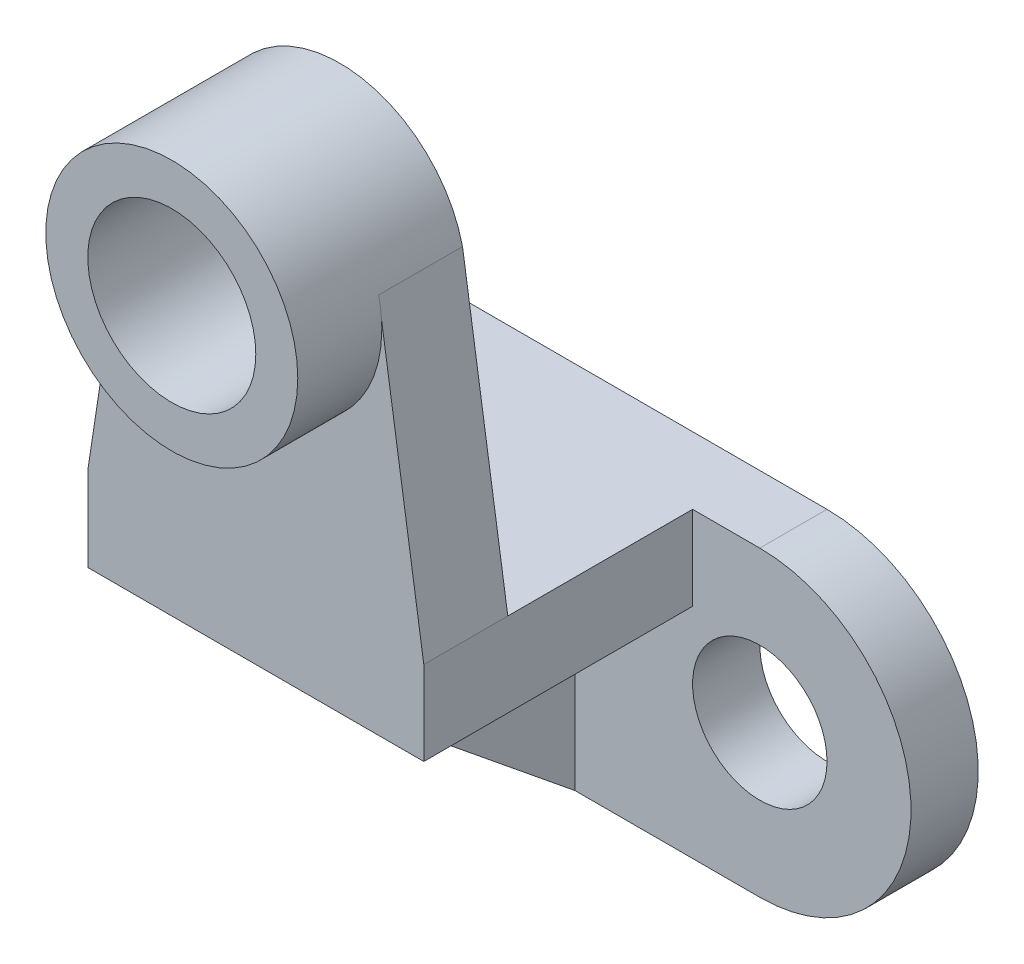
ISO-10303-21;
HEADER;
FILE_DESCRIPTION(('STEP AP214'),'2;1');
FILE_NAME('part.step','',(''),(''),'','','');
FILE_SCHEMA(('AUTOMOTIVE_DESIGN { 1 0 10303 214 1 1 1 1 }'));
ENDSEC;
DATA;
#1=APPLICATION_CONTEXT('core data for automotive mechanical design processes');
#2=APPLICATION_PROTOCOL_DEFINITION('international standard','automotive_design',2000,#1);
#3=PRODUCT_CONTEXT('',#1,'mechanical');
#4=PRODUCT('Part','Part','',(#3));
#5=PRODUCT_RELATED_PRODUCT_CATEGORY('part','',(#4));
#6=PRODUCT_DEFINITION_FORMATION('','',#4);
#7=PRODUCT_DEFINITION_CONTEXT('part definition',#1,'design');
#8=PRODUCT_DEFINITION('design','',#6,#7);
#9=PRODUCT_DEFINITION_SHAPE('','',#8);
#10=(LENGTH_UNIT() NAMED_UNIT(*) SI_UNIT(.MILLI.,.METRE.));
#11=(NAMED_UNIT(*) PLANE_ANGLE_UNIT() SI_UNIT($,.RADIAN.));
#12=(NAMED_UNIT(*) SI_UNIT($,.STERADIAN.) SOLID_ANGLE_UNIT());
#13=UNCERTAINTY_MEASURE_WITH_UNIT(LENGTH_MEASURE(1.E-05),#10,'distance_accuracy_value','');
#14=(GEOMETRIC_REPRESENTATION_CONTEXT(3) GLOBAL_UNCERTAINTY_ASSIGNED_CONTEXT((#13)) GLOBAL_UNIT_ASSIGNED_CONTEXT((#10,
#11,#12)) REPRESENTATION_CONTEXT('',''));
#15=CARTESIAN_POINT('',(0.,0.,0.));
#16=DIRECTION('',(0.,0.,1.));
#17=DIRECTION('',(1.,0.,0.));
#18=AXIS2_PLACEMENT_3D('',#15,#16,#17);
#19=CARTESIAN_POINT('',(8.,8.,40.));
#20=DIRECTION('',(0.,-0.776114000116266,0.630592625094466));
#21=DIRECTION('',(0.,-0.630592625094466,-0.776114000116266));
#22=AXIS2_PLACEMENT_3D('',#19,#20,#21);
#23=PLANE('',#22);
#24=DIRECTION('',(0.,0.630592625094466,0.776114000116266));
#25=VECTOR('',#24,1.);
#26=CARTESIAN_POINT('',(22.,-18.,8.));
#27=LINE('',#26,#25);
#28=CARTESIAN_POINT('',(22.,-18.,8.));
#29=VERTEX_POINT('',#28);
#30=CARTESIAN_POINT('',(22.,8.,40.));
#31=VERTEX_POINT('',#30);
#32=EDGE_CURVE('E63',#29,#31,#27,.T.);
#33=ORIENTED_EDGE('',*,*,#32,.F.);
#34=DIRECTION('',(1.,0.,0.));
#35=VECTOR('',#34,1.);
#36=CARTESIAN_POINT('',(8.,-18.,8.));
#37=LINE('',#36,#35);
#38=CARTESIAN_POINT('',(34.,-18.,8.));
#39=VERTEX_POINT('',#38);
#40=EDGE_CURVE('E194',#29,#39,#37,.T.);
#41=ORIENTED_EDGE('',*,*,#40,.T.);
#42=DIRECTION('',(0.,-0.630592625094466,-0.776114000116266));
#43=VECTOR('',#42,1.);
#44=CARTESIAN_POINT('',(34.,-18.,8.));
#45=LINE('',#44,#43);
#46=CARTESIAN_POINT('',(34.,8.,40.));
#47=VERTEX_POINT('',#46);
#48=EDGE_CURVE('E181',#47,#39,#45,.T.);
#49=ORIENTED_EDGE('',*,*,#48,.F.);
#50=DIRECTION('',(1.,0.,0.));
#51=VECTOR('',#50,1.);
#52=CARTESIAN_POINT('',(8.,8.,40.));
#53=LINE('',#52,#51);
#54=EDGE_CURVE('E75',#31,#47,#53,.T.);
#55=ORIENTED_EDGE('',*,*,#54,.F.);
#56=EDGE_LOOP('',(#33,#41,#49,#55));
#57=FACE_BOUND('',#56,.T.);
#58=ADVANCED_FACE('F50',(#57),#23,.T.);
#59=CARTESIAN_POINT('',(0.,0.,8.));
#60=DIRECTION('',(0.,0.,1.));
#61=DIRECTION('',(1.,0.,0.));
#62=AXIS2_PLACEMENT_3D('',#59,#60,#61);
#63=PLANE('',#62);
#64=DIRECTION('',(0.,1.,0.));
#65=VECTOR('',#64,1.);
#66=CARTESIAN_POINT('',(48.,8.,8.));
#67=LINE('',#66,#65);
#68=CARTESIAN_POINT('',(48.,8.00000000000001,8.));
#69=VERTEX_POINT('',#68);
#70=CARTESIAN_POINT('',(48.,18.,8.));
#71=VERTEX_POINT('',#70);
#72=EDGE_CURVE('E235',#69,#71,#67,.T.);
#73=ORIENTED_EDGE('',*,*,#72,.F.);
#74=DIRECTION('',(1.,0.,0.));
#75=VECTOR('',#74,1.);
#76=CARTESIAN_POINT('',(34.,8.00000000000001,8.));
#77=LINE('',#76,#75);
#78=CARTESIAN_POINT('',(34.,8.00000000000001,8.));
#79=VERTEX_POINT('',#78);
#80=EDGE_CURVE('E186',#79,#69,#77,.T.);
#81=ORIENTED_EDGE('',*,*,#80,.F.);
#82=DIRECTION('',(0.,1.,0.));
#83=VECTOR('',#82,1.);
#84=CARTESIAN_POINT('',(34.,8.00000000000001,8.));
#85=LINE('',#84,#83);
#86=EDGE_CURVE('E183',#39,#79,#85,.T.);
#87=ORIENTED_EDGE('',*,*,#86,.F.);
#88=DIRECTION('',(1.,0.,0.));
#89=VECTOR('',#88,1.);
#90=CARTESIAN_POINT('',(56.,-18.,8.));
#91=LINE('',#90,#89);
#92=CARTESIAN_POINT('',(56.,-18.,8.));
#93=VERTEX_POINT('',#92);
#94=EDGE_CURVE('E264',#39,#93,#91,.T.);
#95=ORIENTED_EDGE('',*,*,#94,.T.);
#96=CARTESIAN_POINT('',(56.,0.,8.));
#97=DIRECTION('',(0.,0.,1.));
#98=DIRECTION('',(1.,0.,0.));
#99=AXIS2_PLACEMENT_3D('',#96,#97,#98);
#100=CIRCLE('',#99,18.);
#101=CARTESIAN_POINT('',(56.,18.,8.));
#102=VERTEX_POINT('',#101);
#103=EDGE_CURVE('E263',#93,#102,#100,.T.);
#104=ORIENTED_EDGE('',*,*,#103,.T.);
#105=DIRECTION('',(-1.,0.,0.));
#106=VECTOR('',#105,1.);
#107=CARTESIAN_POINT('',(0.,18.,8.));
#108=LINE('',#107,#106);
#109=EDGE_CURVE('E270',#102,#71,#108,.T.);
#110=ORIENTED_EDGE('',*,*,#109,.T.);
#111=EDGE_LOOP('',(#73,#81,#87,#95,#104,#110));
#112=FACE_BOUND('',#111,.T.);
#113=CARTESIAN_POINT('',(56.,0.,8.));
#114=DIRECTION('',(0.,0.,1.));
#115=DIRECTION('',(1.,0.,0.));
#116=AXIS2_PLACEMENT_3D('',#113,#114,#115);
#117=CIRCLE('',#116,8.00000000000001);
#118=CARTESIAN_POINT('',(64.,0.,8.));
#119=VERTEX_POINT('',#118);
#120=EDGE_CURVE('E250',#119,#119,#117,.T.);
#121=ORIENTED_EDGE('',*,*,#120,.F.);
#122=EDGE_LOOP('',(#121));
#123=FACE_BOUND('',#122,.T.);
#124=ADVANCED_FACE('F311',(#112,#123),#63,.T.);
#125=CARTESIAN_POINT('',(0.,18.,8.));
#126=DIRECTION('',(0.,-1.,0.));
#127=DIRECTION('',(1.,0.,0.));
#128=AXIS2_PLACEMENT_3D('',#125,#126,#127);
#129=PLANE('',#128);
#130=DIRECTION('',(-1.,0.,0.));
#131=VECTOR('',#130,1.);
#132=CARTESIAN_POINT('',(0.,18.,30.));
#133=LINE('',#132,#131);
#134=CARTESIAN_POINT('',(48.,18.,30.));
#135=VERTEX_POINT('',#134);
#136=CARTESIAN_POINT('',(8.,18.,30.));
#137=VERTEX_POINT('',#136);
#138=EDGE_CURVE('E217',#135,#137,#133,.T.);
#139=ORIENTED_EDGE('',*,*,#138,.F.);
#140=DIRECTION('',(0.,0.,-1.));
#141=VECTOR('',#140,1.);
#142=CARTESIAN_POINT('',(48.,18.,40.));
#143=LINE('',#142,#141);
#144=EDGE_CURVE('E238',#135,#71,#143,.T.);
#145=ORIENTED_EDGE('',*,*,#144,.T.);
#146=ORIENTED_EDGE('',*,*,#109,.F.);
#147=DIRECTION('',(0.,0.,-1.));
#148=VECTOR('',#147,1.);
#149=CARTESIAN_POINT('',(56.,18.,8.));
#150=LINE('',#149,#148);
#151=CARTESIAN_POINT('',(56.,18.,0.));
#152=VERTEX_POINT('',#151);
#153=EDGE_CURVE('E282',#102,#152,#150,.T.);
#154=ORIENTED_EDGE('',*,*,#153,.T.);
#155=DIRECTION('',(-1.,0.,0.));
#156=VECTOR('',#155,1.);
#157=CARTESIAN_POINT('',(0.,18.,0.));
#158=LINE('',#157,#156);
#159=CARTESIAN_POINT('',(0.,18.,0.));
#160=VERTEX_POINT('',#159);
#161=EDGE_CURVE('E265',#152,#160,#158,.T.);
#162=ORIENTED_EDGE('',*,*,#161,.T.);
#163=DIRECTION('',(0.,0.,-1.));
#164=VECTOR('',#163,1.);
#165=CARTESIAN_POINT('',(0.,18.,8.));
#166=LINE('',#165,#164);
#167=CARTESIAN_POINT('',(0.,18.,8.));
#168=VERTEX_POINT('',#167);
#169=EDGE_CURVE('E272',#168,#160,#166,.T.);
#170=ORIENTED_EDGE('',*,*,#169,.F.);
#171=CARTESIAN_POINT('',(8.,18.,8.));
#172=VERTEX_POINT('',#171);
#173=EDGE_CURVE('E266',#172,#168,#108,.T.);
#174=ORIENTED_EDGE('',*,*,#173,.F.);
#175=DIRECTION('',(0.,0.,-1.));
#176=VECTOR('',#175,1.);
#177=CARTESIAN_POINT('',(8.,18.,40.));
#178=LINE('',#177,#176);
#179=EDGE_CURVE('E243',#137,#172,#178,.T.);
#180=ORIENTED_EDGE('',*,*,#179,.F.);
#181=EDGE_LOOP('',(#139,#145,#146,#154,#162,#170,#174,#180));
#182=FACE_BOUND('',#181,.T.);
#183=ADVANCED_FACE('F306',(#182),#129,.F.);
#184=CARTESIAN_POINT('',(0.,0.,8.));
#185=DIRECTION('',(0.,0.,-1.));
#186=DIRECTION('',(-1.,0.,0.));
#187=AXIS2_PLACEMENT_3D('',#184,#185,#186);
#188=CYLINDRICAL_SURFACE('',#187,18.);
#189=CARTESIAN_POINT('',(0.,0.,0.));
#190=DIRECTION('',(0.,0.,1.));
#191=DIRECTION('',(1.,0.,0.));
#192=AXIS2_PLACEMENT_3D('',#189,#190,#191);
#193=CIRCLE('',#192,18.);
#194=CARTESIAN_POINT('',(0.,-18.,0.));
#195=VERTEX_POINT('',#194);
#196=EDGE_CURVE('E252',#160,#195,#193,.T.);
#197=ORIENTED_EDGE('',*,*,#196,.T.);
#198=DIRECTION('',(0.,0.,-1.));
#199=VECTOR('',#198,1.);
#200=CARTESIAN_POINT('',(0.,-18.,8.));
#201=LINE('',#200,#199);
#202=CARTESIAN_POINT('',(0.,-18.,8.));
#203=VERTEX_POINT('',#202);
#204=EDGE_CURVE('E51',#203,#195,#201,.T.);
#205=ORIENTED_EDGE('',*,*,#204,.F.);
#206=CARTESIAN_POINT('',(0.,0.,8.));
#207=DIRECTION('',(0.,0.,1.));
#208=DIRECTION('',(1.,0.,0.));
#209=AXIS2_PLACEMENT_3D('',#206,#207,#208);
#210=CIRCLE('',#209,18.);
#211=EDGE_CURVE('E258',#168,#203,#210,.T.);
#212=ORIENTED_EDGE('',*,*,#211,.F.);
#213=ORIENTED_EDGE('',*,*,#169,.T.);
#214=EDGE_LOOP('',(#197,#205,#212,#213));
#215=FACE_BOUND('',#214,.T.);
#216=ADVANCED_FACE('F47',(#215),#188,.T.);
#217=CARTESIAN_POINT('',(56.,-18.,8.));
#218=DIRECTION('',(0.,1.,0.));
#219=DIRECTION('',(-1.,0.,0.));
#220=AXIS2_PLACEMENT_3D('',#217,#218,#219);
#221=PLANE('',#220);
#222=DIRECTION('',(1.,0.,0.));
#223=VECTOR('',#222,1.);
#224=CARTESIAN_POINT('',(56.,-18.,0.));
#225=LINE('',#224,#223);
#226=CARTESIAN_POINT('',(56.,-18.,0.));
#227=VERTEX_POINT('',#226);
#228=EDGE_CURVE('E274',#195,#227,#225,.T.);
#229=ORIENTED_EDGE('',*,*,#228,.T.);
#230=DIRECTION('',(0.,0.,-1.));
#231=VECTOR('',#230,1.);
#232=CARTESIAN_POINT('',(56.,-18.,8.));
#233=LINE('',#232,#231);
#234=EDGE_CURVE('E285',#93,#227,#233,.T.);
#235=ORIENTED_EDGE('',*,*,#234,.F.);
#236=ORIENTED_EDGE('',*,*,#94,.F.);
#237=ORIENTED_EDGE('',*,*,#40,.F.);
#238=EDGE_CURVE('E176',#203,#29,#91,.T.);
#239=ORIENTED_EDGE('',*,*,#238,.F.);
#240=ORIENTED_EDGE('',*,*,#204,.T.);
#241=EDGE_LOOP('',(#229,#235,#236,#237,#239,#240));
#242=FACE_BOUND('',#241,.T.);
#243=ADVANCED_FACE('F292',(#242),#221,.F.);
#244=CARTESIAN_POINT('',(56.,0.,8.));
#245=DIRECTION('',(0.,0.,-1.));
#246=DIRECTION('',(-1.,0.,0.));
#247=AXIS2_PLACEMENT_3D('',#244,#245,#246);
#248=CYLINDRICAL_SURFACE('',#247,18.);
#249=CARTESIAN_POINT('',(56.,0.,0.));
#250=DIRECTION('',(0.,0.,1.));
#251=DIRECTION('',(1.,0.,0.));
#252=AXIS2_PLACEMENT_3D('',#249,#250,#251);
#253=CIRCLE('',#252,18.);
#254=EDGE_CURVE('E277',#227,#152,#253,.T.);
#255=ORIENTED_EDGE('',*,*,#254,.T.);
#256=ORIENTED_EDGE('',*,*,#153,.F.);
#257=ORIENTED_EDGE('',*,*,#103,.F.);
#258=ORIENTED_EDGE('',*,*,#234,.T.);
#259=EDGE_LOOP('',(#255,#256,#257,#258));
#260=FACE_BOUND('',#259,.T.);
#261=ADVANCED_FACE('F305',(#260),#248,.T.);
#262=CARTESIAN_POINT('',(0.,0.,8.));
#263=DIRECTION('',(0.,0.,1.));
#264=DIRECTION('',(1.,0.,0.));
#265=AXIS2_PLACEMENT_3D('',#262,#263,#264);
#266=CIRCLE('',#265,8.);
#267=CARTESIAN_POINT('',(8.,0.,8.));
#268=VERTEX_POINT('',#267);
#269=EDGE_CURVE('E255',#268,#268,#266,.T.);
#270=ORIENTED_EDGE('',*,*,#269,.F.);
#271=EDGE_LOOP('',(#270));
#272=FACE_BOUND('',#271,.T.);
#273=ORIENTED_EDGE('',*,*,#238,.T.);
#274=DIRECTION('',(0.,-1.,0.));
#275=VECTOR('',#274,1.);
#276=CARTESIAN_POINT('',(22.,8.,8.));
#277=LINE('',#276,#275);
#278=CARTESIAN_POINT('',(22.,8.,8.));
#279=VERTEX_POINT('',#278);
#280=EDGE_CURVE('E167',#279,#29,#277,.T.);
#281=ORIENTED_EDGE('',*,*,#280,.F.);
#282=DIRECTION('',(-1.,0.,0.));
#283=VECTOR('',#282,1.);
#284=CARTESIAN_POINT('',(22.,8.,8.));
#285=LINE('',#284,#283);
#286=CARTESIAN_POINT('',(8.,8.,8.));
#287=VERTEX_POINT('',#286);
#288=EDGE_CURVE('E157',#279,#287,#285,.T.);
#289=ORIENTED_EDGE('',*,*,#288,.T.);
#290=DIRECTION('',(0.,-1.,0.));
#291=VECTOR('',#290,1.);
#292=CARTESIAN_POINT('',(8.,18.,8.));
#293=LINE('',#292,#291);
#294=EDGE_CURVE('E227',#172,#287,#293,.T.);
#295=ORIENTED_EDGE('',*,*,#294,.F.);
#296=ORIENTED_EDGE('',*,*,#173,.T.);
#297=ORIENTED_EDGE('',*,*,#211,.T.);
#298=EDGE_LOOP('',(#273,#281,#289,#295,#296,#297));
#299=FACE_BOUND('',#298,.T.);
#300=ADVANCED_FACE('F172',(#272,#299),#63,.T.);
#301=CARTESIAN_POINT('',(0.,0.,0.));
#302=DIRECTION('',(0.,0.,1.));
#303=DIRECTION('',(1.,0.,0.));
#304=AXIS2_PLACEMENT_3D('',#301,#302,#303);
#305=PLANE('',#304);
#306=CARTESIAN_POINT('',(0.,0.,0.));
#307=DIRECTION('',(0.,0.,1.));
#308=DIRECTION('',(1.,0.,0.));
#309=AXIS2_PLACEMENT_3D('',#306,#307,#308);
#310=CIRCLE('',#309,8.);
#311=CARTESIAN_POINT('',(8.,0.,0.));
#312=VERTEX_POINT('',#311);
#313=EDGE_CURVE('E247',#312,#312,#310,.T.);
#314=ORIENTED_EDGE('',*,*,#313,.T.);
#315=EDGE_LOOP('',(#314));
#316=FACE_BOUND('',#315,.T.);
#317=CARTESIAN_POINT('',(56.,0.,0.));
#318=DIRECTION('',(0.,0.,1.));
#319=DIRECTION('',(1.,0.,0.));
#320=AXIS2_PLACEMENT_3D('',#317,#318,#319);
#321=CIRCLE('',#320,8.00000000000001);
#322=CARTESIAN_POINT('',(64.,0.,0.));
#323=VERTEX_POINT('',#322);
#324=EDGE_CURVE('E253',#323,#323,#321,.T.);
#325=ORIENTED_EDGE('',*,*,#324,.T.);
#326=EDGE_LOOP('',(#325));
#327=FACE_BOUND('',#326,.T.);
#328=ORIENTED_EDGE('',*,*,#196,.F.);
#329=ORIENTED_EDGE('',*,*,#161,.F.);
#330=ORIENTED_EDGE('',*,*,#254,.F.);
#331=ORIENTED_EDGE('',*,*,#228,.F.);
#332=EDGE_LOOP('',(#328,#329,#330,#331));
#333=FACE_BOUND('',#332,.T.);
#334=ADVANCED_FACE('F297',(#316,#327,#333),#305,.F.);
#335=CARTESIAN_POINT('',(56.,0.,0.));
#336=DIRECTION('',(0.,0.,1.));
#337=DIRECTION('',(1.,0.,0.));
#338=AXIS2_PLACEMENT_3D('',#335,#336,#337);
#339=CYLINDRICAL_SURFACE('',#338,8.00000000000001);
#340=ORIENTED_EDGE('',*,*,#324,.F.);
#341=EDGE_LOOP('',(#340));
#342=FACE_BOUND('',#341,.T.);
#343=ORIENTED_EDGE('',*,*,#120,.T.);
#344=EDGE_LOOP('',(#343));
#345=FACE_BOUND('',#344,.T.);
#346=ADVANCED_FACE('F408',(#342,#345),#339,.F.);
#347=CARTESIAN_POINT('',(0.,0.,0.));
#348=DIRECTION('',(0.,0.,1.));
#349=DIRECTION('',(1.,0.,0.));
#350=AXIS2_PLACEMENT_3D('',#347,#348,#349);
#351=CYLINDRICAL_SURFACE('',#350,8.);
#352=ORIENTED_EDGE('',*,*,#313,.F.);
#353=EDGE_LOOP('',(#352));
#354=FACE_BOUND('',#353,.T.);
#355=ORIENTED_EDGE('',*,*,#269,.T.);
#356=EDGE_LOOP('',(#355));
#357=FACE_BOUND('',#356,.T.);
#358=ADVANCED_FACE('F409',(#354,#357),#351,.F.);
#359=CARTESIAN_POINT('',(8.,18.,40.));
#360=DIRECTION('',(1.,0.,0.));
#361=DIRECTION('',(0.,0.,-1.));
#362=AXIS2_PLACEMENT_3D('',#359,#360,#361);
#363=PLANE('',#362);
#364=ORIENTED_EDGE('',*,*,#294,.T.);
#365=DIRECTION('',(0.,0.,-1.));
#366=VECTOR('',#365,1.);
#367=CARTESIAN_POINT('',(8.,8.,40.));
#368=LINE('',#367,#366);
#369=CARTESIAN_POINT('',(8.,8.,40.));
#370=VERTEX_POINT('',#369);
#371=EDGE_CURVE('E165',#370,#287,#368,.T.);
#372=ORIENTED_EDGE('',*,*,#371,.F.);
#373=DIRECTION('',(0.,-1.,0.));
#374=VECTOR('',#373,1.);
#375=CARTESIAN_POINT('',(8.,18.,40.));
#376=LINE('',#375,#374);
#377=CARTESIAN_POINT('',(8.,18.,40.));
#378=VERTEX_POINT('',#377);
#379=EDGE_CURVE('E230',#378,#370,#376,.T.);
#380=ORIENTED_EDGE('',*,*,#379,.F.);
#381=EDGE_CURVE('E242',#378,#137,#178,.T.);
#382=ORIENTED_EDGE('',*,*,#381,.T.);
#383=ORIENTED_EDGE('',*,*,#179,.T.);
#384=EDGE_LOOP('',(#364,#372,#380,#382,#383));
#385=FACE_BOUND('',#384,.T.);
#386=ADVANCED_FACE('F318',(#385),#363,.F.);
#387=CARTESIAN_POINT('',(48.,8.,40.));
#388=DIRECTION('',(-1.,0.,0.));
#389=DIRECTION('',(0.,0.,1.));
#390=AXIS2_PLACEMENT_3D('',#387,#388,#389);
#391=PLANE('',#390);
#392=DIRECTION('',(0.,1.,0.));
#393=VECTOR('',#392,1.);
#394=CARTESIAN_POINT('',(48.,8.,40.));
#395=LINE('',#394,#393);
#396=CARTESIAN_POINT('',(48.,8.,40.));
#397=VERTEX_POINT('',#396);
#398=CARTESIAN_POINT('',(48.,18.,40.));
#399=VERTEX_POINT('',#398);
#400=EDGE_CURVE('E232',#397,#399,#395,.T.);
#401=ORIENTED_EDGE('',*,*,#400,.F.);
#402=DIRECTION('',(0.,0.,1.));
#403=VECTOR('',#402,1.);
#404=CARTESIAN_POINT('',(48.,8.,40.));
#405=LINE('',#404,#403);
#406=EDGE_CURVE('E169',#69,#397,#405,.T.);
#407=ORIENTED_EDGE('',*,*,#406,.F.);
#408=ORIENTED_EDGE('',*,*,#72,.T.);
#409=ORIENTED_EDGE('',*,*,#144,.F.);
#410=EDGE_CURVE('E241',#399,#135,#143,.T.);
#411=ORIENTED_EDGE('',*,*,#410,.F.);
#412=EDGE_LOOP('',(#401,#407,#408,#409,#411));
#413=FACE_BOUND('',#412,.T.);
#414=ADVANCED_FACE('F338',(#413),#391,.F.);
#415=CARTESIAN_POINT('',(0.,0.,40.));
#416=DIRECTION('',(0.,0.,1.));
#417=DIRECTION('',(1.,0.,0.));
#418=AXIS2_PLACEMENT_3D('',#415,#416,#417);
#419=PLANE('',#418);
#420=CARTESIAN_POINT('',(28.,50.,40.));
#421=DIRECTION('',(0.,0.,1.));
#422=DIRECTION('',(1.,0.,0.));
#423=AXIS2_PLACEMENT_3D('',#420,#421,#422);
#424=CIRCLE('',#423,15.);
#425=CARTESIAN_POINT('',(13.0411953772836,51.1109294574359,40.));
#426=VERTEX_POINT('',#425);
#427=CARTESIAN_POINT('',(42.9588046227164,51.1109294574359,40.));
#428=VERTEX_POINT('',#427);
#429=EDGE_CURVE('E11',#426,#428,#424,.T.);
#430=ORIENTED_EDGE('',*,*,#429,.F.);
#431=DIRECTION('',(0.15051715913292,0.988607396698282,0.));
#432=VECTOR('',#431,1.);
#433=CARTESIAN_POINT('',(5.14031389517373,-0.782621541308532,40.));
#434=LINE('',#433,#432);
#435=EDGE_CURVE('E212',#378,#426,#434,.T.);
#436=ORIENTED_EDGE('',*,*,#435,.F.);
#437=ORIENTED_EDGE('',*,*,#379,.T.);
#438=EDGE_CURVE('E231',#370,#31,#53,.T.);
#439=ORIENTED_EDGE('',*,*,#438,.T.);
#440=ORIENTED_EDGE('',*,*,#54,.T.);
#441=DIRECTION('',(1.,0.,0.));
#442=VECTOR('',#441,1.);
#443=CARTESIAN_POINT('',(34.,8.,40.));
#444=LINE('',#443,#442);
#445=EDGE_CURVE('E192',#47,#397,#444,.T.);
#446=ORIENTED_EDGE('',*,*,#445,.T.);
#447=ORIENTED_EDGE('',*,*,#400,.T.);
#448=DIRECTION('',(-0.15051715913292,0.988607396698282,0.));
#449=VECTOR('',#448,1.);
#450=CARTESIAN_POINT('',(49.5909828539934,7.55031156222524,40.));
#451=LINE('',#450,#449);
#452=EDGE_CURVE('E216',#399,#428,#451,.T.);
#453=ORIENTED_EDGE('',*,*,#452,.T.);
#454=EDGE_LOOP('',(#430,#436,#437,#439,#440,#446,#447,#453));
#455=FACE_BOUND('',#454,.T.);
#456=ADVANCED_FACE('F320',(#455),#419,.T.);
#457=CARTESIAN_POINT('',(49.5909828539934,7.55031156222524,30.));
#458=DIRECTION('',(0.988607396698282,0.15051715913292,0.));
#459=DIRECTION('',(-0.15051715913292,0.988607396698282,0.));
#460=AXIS2_PLACEMENT_3D('',#457,#458,#459);
#461=PLANE('',#460);
#462=ORIENTED_EDGE('',*,*,#452,.F.);
#463=ORIENTED_EDGE('',*,*,#410,.T.);
#464=DIRECTION('',(-0.15051715913292,0.988607396698282,0.));
#465=VECTOR('',#464,1.);
#466=CARTESIAN_POINT('',(49.5909828539934,7.55031156222524,30.));
#467=LINE('',#466,#465);
#468=CARTESIAN_POINT('',(42.6116266512215,53.3912190441364,30.));
#469=VERTEX_POINT('',#468);
#470=EDGE_CURVE('E210',#135,#469,#467,.T.);
#471=ORIENTED_EDGE('',*,*,#470,.T.);
#472=DIRECTION('',(0.,0.,1.));
#473=VECTOR('',#472,1.);
#474=CARTESIAN_POINT('',(42.6116266512215,53.3912190441364,30.));
#475=LINE('',#474,#473);
#476=CARTESIAN_POINT('',(42.6116266512215,53.3912190441364,40.));
#477=VERTEX_POINT('',#476);
#478=EDGE_CURVE('E220',#469,#477,#475,.T.);
#479=ORIENTED_EDGE('',*,*,#478,.T.);
#480=EDGE_CURVE('E203',#428,#477,#451,.T.);
#481=ORIENTED_EDGE('',*,*,#480,.F.);
#482=EDGE_LOOP('',(#462,#463,#471,#479,#481));
#483=FACE_BOUND('',#482,.T.);
#484=ADVANCED_FACE('F333',(#483),#461,.T.);
#485=CARTESIAN_POINT('',(5.14031389517373,-0.782621541308532,30.));
#486=DIRECTION('',(0.988607396698282,-0.15051715913292,0.));
#487=DIRECTION('',(0.15051715913292,0.988607396698282,0.));
#488=AXIS2_PLACEMENT_3D('',#485,#486,#487);
#489=PLANE('',#488);
#490=ORIENTED_EDGE('',*,*,#435,.T.);
#491=CARTESIAN_POINT('',(13.3883733487785,53.3912190441364,40.));
#492=VERTEX_POINT('',#491);
#493=EDGE_CURVE('E224',#426,#492,#434,.T.);
#494=ORIENTED_EDGE('',*,*,#493,.T.);
#495=DIRECTION('',(0.,0.,1.));
#496=VECTOR('',#495,1.);
#497=CARTESIAN_POINT('',(13.3883733487785,53.3912190441364,30.));
#498=LINE('',#497,#496);
#499=CARTESIAN_POINT('',(13.3883733487785,53.3912190441364,30.));
#500=VERTEX_POINT('',#499);
#501=EDGE_CURVE('E223',#500,#492,#498,.T.);
#502=ORIENTED_EDGE('',*,*,#501,.F.);
#503=DIRECTION('',(0.15051715913292,0.988607396698282,0.));
#504=VECTOR('',#503,1.);
#505=CARTESIAN_POINT('',(5.14031389517373,-0.782621541308532,30.));
#506=LINE('',#505,#504);
#507=EDGE_CURVE('E211',#137,#500,#506,.T.);
#508=ORIENTED_EDGE('',*,*,#507,.F.);
#509=ORIENTED_EDGE('',*,*,#381,.F.);
#510=EDGE_LOOP('',(#490,#494,#502,#508,#509));
#511=FACE_BOUND('',#510,.T.);
#512=ADVANCED_FACE('F327',(#511),#489,.F.);
#513=CARTESIAN_POINT('',(28.,50.,30.));
#514=DIRECTION('',(0.,0.,1.));
#515=DIRECTION('',(1.,0.,0.));
#516=AXIS2_PLACEMENT_3D('',#513,#514,#515);
#517=CYLINDRICAL_SURFACE('',#516,15.);
#518=ORIENTED_EDGE('',*,*,#501,.T.);
#519=EDGE_CURVE('E59',#492,#426,#424,.T.);
#520=ORIENTED_EDGE('',*,*,#519,.T.);
#521=ORIENTED_EDGE('',*,*,#429,.T.);
#522=EDGE_CURVE('E60',#428,#477,#424,.T.);
#523=ORIENTED_EDGE('',*,*,#522,.T.);
#524=ORIENTED_EDGE('',*,*,#478,.F.);
#525=CARTESIAN_POINT('',(28.,50.,30.));
#526=DIRECTION('',(0.,0.,1.));
#527=DIRECTION('',(1.,0.,0.));
#528=AXIS2_PLACEMENT_3D('',#525,#526,#527);
#529=CIRCLE('',#528,15.);
#530=EDGE_CURVE('E208',#469,#500,#529,.T.);
#531=ORIENTED_EDGE('',*,*,#530,.T.);
#532=EDGE_LOOP('',(#518,#520,#521,#523,#524,#531));
#533=FACE_BOUND('',#532,.T.);
#534=CARTESIAN_POINT('',(28.,50.,50.));
#535=DIRECTION('',(0.,0.,1.));
#536=DIRECTION('',(1.,0.,0.));
#537=AXIS2_PLACEMENT_3D('',#534,#535,#536);
#538=CIRCLE('',#537,15.);
#539=CARTESIAN_POINT('',(43.,50.,50.));
#540=VERTEX_POINT('',#539);
#541=EDGE_CURVE('E201',#540,#540,#538,.T.);
#542=ORIENTED_EDGE('',*,*,#541,.F.);
#543=EDGE_LOOP('',(#542));
#544=FACE_BOUND('',#543,.T.);
#545=ADVANCED_FACE('F348',(#533,#544),#517,.T.);
#546=CARTESIAN_POINT('',(0.,0.,30.));
#547=DIRECTION('',(0.,0.,1.));
#548=DIRECTION('',(1.,0.,0.));
#549=AXIS2_PLACEMENT_3D('',#546,#547,#548);
#550=PLANE('',#549);
#551=CARTESIAN_POINT('',(28.,50.,30.));
#552=DIRECTION('',(0.,0.,1.));
#553=DIRECTION('',(1.,0.,0.));
#554=AXIS2_PLACEMENT_3D('',#551,#552,#553);
#555=CIRCLE('',#554,10.);
#556=CARTESIAN_POINT('',(38.,50.,30.));
#557=VERTEX_POINT('',#556);
#558=EDGE_CURVE('E199',#557,#557,#555,.T.);
#559=ORIENTED_EDGE('',*,*,#558,.T.);
#560=EDGE_LOOP('',(#559));
#561=FACE_BOUND('',#560,.T.);
#562=ORIENTED_EDGE('',*,*,#470,.F.);
#563=ORIENTED_EDGE('',*,*,#138,.T.);
#564=ORIENTED_EDGE('',*,*,#507,.T.);
#565=ORIENTED_EDGE('',*,*,#530,.F.);
#566=EDGE_LOOP('',(#562,#563,#564,#565));
#567=FACE_BOUND('',#566,.T.);
#568=ADVANCED_FACE('F331',(#561,#567),#550,.F.);
#569=CARTESIAN_POINT('',(28.,50.,40.));
#570=DIRECTION('',(0.,0.,1.));
#571=DIRECTION('',(1.,0.,0.));
#572=AXIS2_PLACEMENT_3D('',#569,#570,#571);
#573=PLANE('',#572);
#574=ORIENTED_EDGE('',*,*,#522,.F.);
#575=ORIENTED_EDGE('',*,*,#480,.T.);
#576=EDGE_LOOP('',(#574,#575));
#577=FACE_BOUND('',#576,.T.);
#578=ADVANCED_FACE('F355',(#577),#573,.F.);
#579=CARTESIAN_POINT('',(28.,50.,50.));
#580=DIRECTION('',(0.,0.,1.));
#581=DIRECTION('',(1.,0.,0.));
#582=AXIS2_PLACEMENT_3D('',#579,#580,#581);
#583=PLANE('',#582);
#584=CARTESIAN_POINT('',(28.,50.,50.));
#585=DIRECTION('',(0.,0.,1.));
#586=DIRECTION('',(1.,0.,0.));
#587=AXIS2_PLACEMENT_3D('',#584,#585,#586);
#588=CIRCLE('',#587,10.);
#589=CARTESIAN_POINT('',(38.,50.,50.));
#590=VERTEX_POINT('',#589);
#591=EDGE_CURVE('E197',#590,#590,#588,.T.);
#592=ORIENTED_EDGE('',*,*,#591,.F.);
#593=EDGE_LOOP('',(#592));
#594=FACE_BOUND('',#593,.T.);
#595=ORIENTED_EDGE('',*,*,#541,.T.);
#596=EDGE_LOOP('',(#595));
#597=FACE_BOUND('',#596,.T.);
#598=ADVANCED_FACE('F352',(#594,#597),#583,.T.);
#599=ORIENTED_EDGE('',*,*,#493,.F.);
#600=ORIENTED_EDGE('',*,*,#519,.F.);
#601=EDGE_LOOP('',(#599,#600));
#602=FACE_BOUND('',#601,.T.);
#603=ADVANCED_FACE('F357',(#602),#573,.F.);
#604=CARTESIAN_POINT('',(28.,50.,30.));
#605=DIRECTION('',(0.,0.,1.));
#606=DIRECTION('',(1.,0.,0.));
#607=AXIS2_PLACEMENT_3D('',#604,#605,#606);
#608=CYLINDRICAL_SURFACE('',#607,10.);
#609=ORIENTED_EDGE('',*,*,#558,.F.);
#610=EDGE_LOOP('',(#609));
#611=FACE_BOUND('',#610,.T.);
#612=ORIENTED_EDGE('',*,*,#591,.T.);
#613=EDGE_LOOP('',(#612));
#614=FACE_BOUND('',#613,.T.);
#615=ADVANCED_FACE('F368',(#611,#614),#608,.F.);
#616=CARTESIAN_POINT('',(34.,8.,40.));
#617=DIRECTION('',(0.,1.,0.));
#618=DIRECTION('',(0.,0.,1.));
#619=AXIS2_PLACEMENT_3D('',#616,#617,#618);
#620=PLANE('',#619);
#621=ORIENTED_EDGE('',*,*,#406,.T.);
#622=ORIENTED_EDGE('',*,*,#445,.F.);
#623=DIRECTION('',(0.,0.,1.));
#624=VECTOR('',#623,1.);
#625=CARTESIAN_POINT('',(34.,8.,40.));
#626=LINE('',#625,#624);
#627=EDGE_CURVE('E190',#79,#47,#626,.T.);
#628=ORIENTED_EDGE('',*,*,#627,.F.);
#629=ORIENTED_EDGE('',*,*,#80,.T.);
#630=EDGE_LOOP('',(#621,#622,#628,#629));
#631=FACE_BOUND('',#630,.T.);
#632=ADVANCED_FACE('F341',(#631),#620,.F.);
#633=CARTESIAN_POINT('',(34.,0.,0.));
#634=DIRECTION('',(1.,0.,0.));
#635=DIRECTION('',(0.,0.,-1.));
#636=AXIS2_PLACEMENT_3D('',#633,#634,#635);
#637=PLANE('',#636);
#638=ORIENTED_EDGE('',*,*,#48,.T.);
#639=ORIENTED_EDGE('',*,*,#86,.T.);
#640=ORIENTED_EDGE('',*,*,#627,.T.);
#641=EDGE_LOOP('',(#638,#639,#640));
#642=FACE_BOUND('',#641,.T.);
#643=ADVANCED_FACE('F387',(#642),#637,.T.);
#644=CARTESIAN_POINT('',(22.,8.,40.));
#645=DIRECTION('',(0.,1.,0.));
#646=DIRECTION('',(0.,0.,1.));
#647=AXIS2_PLACEMENT_3D('',#644,#645,#646);
#648=PLANE('',#647);
#649=ORIENTED_EDGE('',*,*,#371,.T.);
#650=ORIENTED_EDGE('',*,*,#288,.F.);
#651=DIRECTION('',(0.,0.,-1.));
#652=VECTOR('',#651,1.);
#653=CARTESIAN_POINT('',(22.,8.,40.));
#654=LINE('',#653,#652);
#655=EDGE_CURVE('E162',#31,#279,#654,.T.);
#656=ORIENTED_EDGE('',*,*,#655,.F.);
#657=ORIENTED_EDGE('',*,*,#438,.F.);
#658=EDGE_LOOP('',(#649,#650,#656,#657));
#659=FACE_BOUND('',#658,.T.);
#660=ADVANCED_FACE('F163',(#659),#648,.F.);
#661=CARTESIAN_POINT('',(22.,0.,0.));
#662=DIRECTION('',(1.,0.,0.));
#663=DIRECTION('',(0.,0.,-1.));
#664=AXIS2_PLACEMENT_3D('',#661,#662,#663);
#665=PLANE('',#664);
#666=ORIENTED_EDGE('',*,*,#32,.T.);
#667=ORIENTED_EDGE('',*,*,#655,.T.);
#668=ORIENTED_EDGE('',*,*,#280,.T.);
#669=EDGE_LOOP('',(#666,#667,#668));
#670=FACE_BOUND('',#669,.T.);
#671=ADVANCED_FACE('F175',(#670),#665,.F.);
#672=CLOSED_SHELL('',(#58,#124,#183,#216,#243,#261,#300,#334,#346,#358,#386,#414,#456,#484,#512,
#545,#568,#578,#598,#603,#615,#632,#643,#660,#671));
#673=MANIFOLD_SOLID_BREP('B2',#672);
#674=ADVANCED_BREP_SHAPE_REPRESENTATION('',(#18,#673),#14);
#675=SHAPE_DEFINITION_REPRESENTATION(#9,#674);
ENDSEC;
END-ISO-10303-21;
